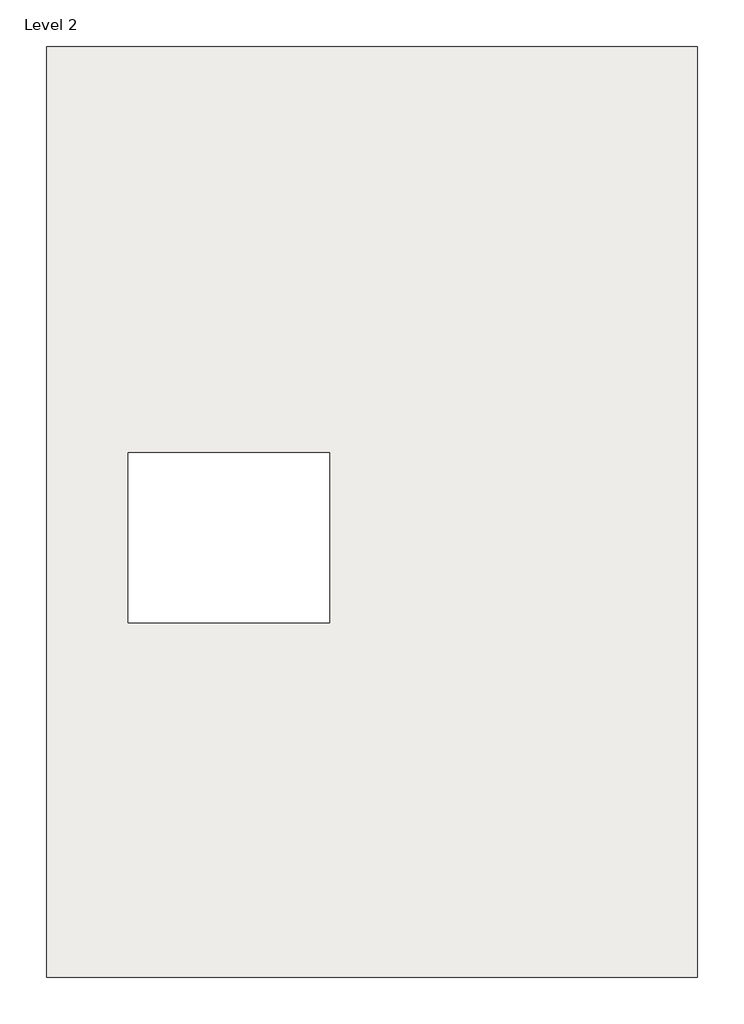
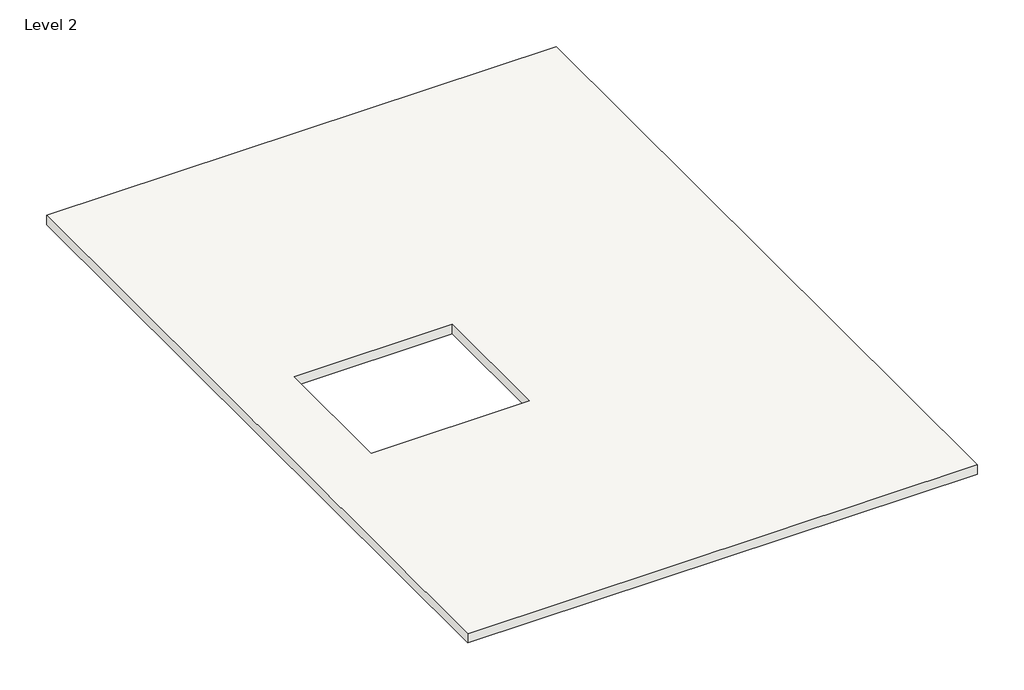
# One storey, incomplete: 1 roof.
"""IFC4 building model written with IfcOpenShell, lengths in millimetres."""

from ifc_helpers import new_model, si_unit, frame, origin, place, context, project, spatial, polyline, outline, extrude, element, save

model = new_model("IFC4")

# Units and contexts
model_context = context("Model", 3, world=origin())
ifc_project = project(units=[si_unit("LENGTHUNIT", "METRE", prefix="MILLI")], contexts=[model_context])

# Site, building, storey
site = spatial("IfcSite", under=ifc_project)
building = spatial("IfcBuilding", under=site)
storey = spatial("IfcBuildingStorey", under=building, Name="Level 2", Elevation=3048.0)

# Roof
placement = place(None, origin())
element("IfcRoof", 1, ObjectType="Generic - 12\"", at=placement, inside=storey, context=model_context, shape_type="SweptSolid", body=[
    extrude(outline(polyline([(-5216.1449167, -5508.2570853), (-5216.1449167, 5769.3429147), (2670.5550833, 5769.3429147), (2670.5550833, -5508.2570853), (-5216.1449167, -5508.2570853)]), holes=[polyline([(-1783.4132248, 848.0929147), (-4225.5449167, 848.0929147), (-4225.5449167, -1209.3070853), (-1783.4132248, -1209.3070853), (-1783.4132248, 848.0929147)])]), frame((0.0, 0.0, 3048.0), z_axis=(0.0, 0.0, 1.0), x_axis=(1.0, 0.0, 0.0)), (0.0, 0.0, 1.0), 152.4),
])

save(model, "model.ifc")

# Revit data of these elements
# Type "Generic - 12\""
#   Assembly Code = "B1020"
#   Layers, outside or top first: 0' - 6" no material (function 1)
# Element 1 (IfcRoof, "Generic - 12\"")
#   built-in parameter 1001705 = 10.5 (stored number, unit not read)
#   built-in parameter 1001710 = 33615
#   Phase Created = New Construction
#   Materials on its faces: "Default Roof", "Wood Planks"
# Materials
#   "Default Roof": colour RGB 88 101 114, transparency 0, Cost = 0
#   "Wood Planks": class "Wood", colour RGB 193 160 115, transparency 0, Description = "Physical material.", Cost = 0
